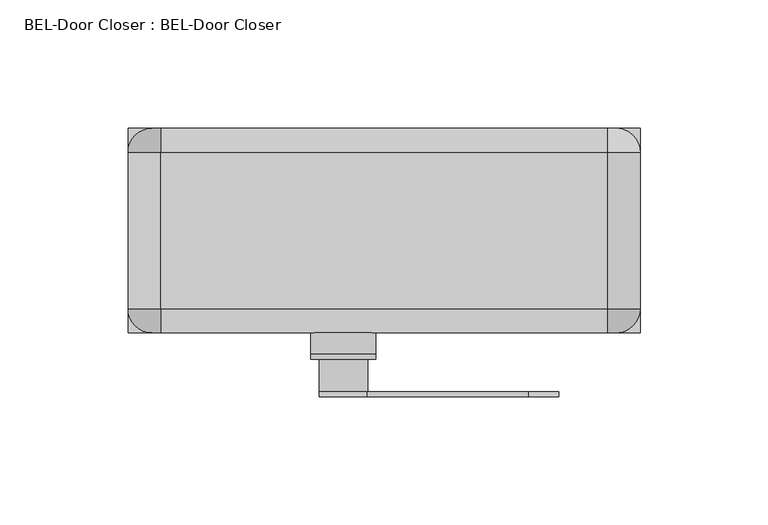
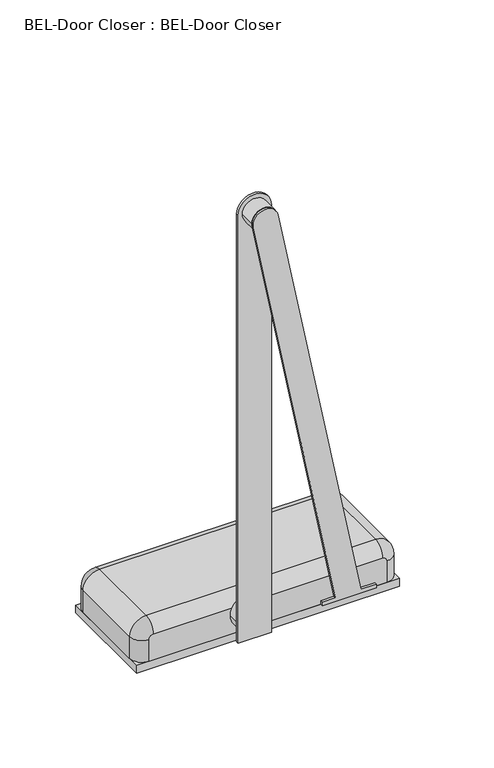
"""IFC4 building model written with IfcOpenShell, lengths in millimetres: proxy geometry, BEL-Door Closer : BEL-Door Closer."""

from ifc_helpers import new_model, si_unit, point, frame, frame_2d, origin, origin_with_axes, place, context, project, spatial, polyline, circle_curve, ellipse_curve, trimmed, segment, composite_curve, outline, extrude, source, transform, mapped, element, save
from ifc_brep_helpers import plane_surface, cylinder_surface, revolved_surface, advanced_brep


def bel_door_closer_bel_door_closer_f210e2f3(model_context):
    return source(origin(), model_context, "Body", "SolidModel", [
        extrude(outline(composite_curve([segment(trimmed(circle_curve(frame_2d((349.25, -273.05)), 9.525), [point((349.25, -282.575))], [point((349.25, -263.525))], False, "CARTESIAN"), True, "CONTINUOUS"), segment(trimmed(circle_curve(frame_2d((349.25, -273.05)), 9.525), [point((349.25, -263.525))], [point((349.25, -282.575))], False, "CARTESIAN"), True, "CONTINUOUS")], self_intersect=False)), frame((0.0, -45.1416667, 0.0), z_axis=(0.0, 1.0, 0.0), x_axis=(0.0, 0.0, 1.0)), (0.0, 0.0, 1.0), 12.5),
        extrude(outline(composite_curve([segment(trimmed(circle_curve(frame_2d((349.25, -273.0495842)), 9.5247276), [point((351.0696907, -263.7002975))], [point((347.4303363, -282.3988762))], False, "CARTESIAN"), True, "CONTINUOUS"), segment(polyline([(347.4303363, -282.3988762), (27.7698622, -220.1829834), (27.7542297, -229.9055371), (24.954228, -229.901035), (25.0199942, -188.9982584), (27.81999, -189.0027604), (27.8010501, -200.7822813), (351.0696907, -263.7002975)]), True, "CONTINUOUS")], self_intersect=False)), frame((0.0, -47.225, 0.0), z_axis=(0.0, 1.0, 0.0), x_axis=(0.0, 0.0, 1.0)), (0.0, 0.0, 1.0), 2.0833333),
        extrude(outline(composite_curve([segment(polyline([(5.475, -260.35), (349.25, -260.35)]), True, "CONTINUOUS"), segment(trimmed(circle_curve(frame_2d((349.25, -273.05)), 12.7), [point((349.25, -260.35))], [point((349.25, -285.75))], False, "CARTESIAN"), True, "CONTINUOUS"), segment(polyline([(349.25, -285.75), (5.475, -285.75), (5.475, -260.35)]), True, "CONTINUOUS")], self_intersect=False)), frame((0.0, -32.6416667, 0.0), z_axis=(0.0, 1.0, 0.0), x_axis=(0.0, 0.0, 1.0)), (0.0, 0.0, 1.0), 2.0833333),
        extrude(outline(composite_curve([segment(trimmed(circle_curve(frame_2d((21.35, -273.05)), 12.7), [point((21.35, -285.75))], [point((21.35, -260.35))], False, "CARTESIAN"), True, "CONTINUOUS"), segment(trimmed(circle_curve(frame_2d((21.35, -273.05)), 12.7), [point((21.35, -260.35))], [point((21.35, -285.75))], False, "CARTESIAN"), True, "CONTINUOUS")], self_intersect=False)), frame((0.0, -30.5583333, 0.0), z_axis=(0.0, 1.0, 0.0), x_axis=(0.0, 0.0, 1.0)), (0.0, 0.0, 1.0), 8.3333333),
        advanced_brep(
        [(-344.4875, -12.7, 36.35), (-169.8875, -12.7, 36.35), (-169.8875, 48.25, 36.35), (-344.4875, 48.25, 36.35), (-157.1875, -12.7, 6.35), (-166.7125, -22.225, 6.35), (-347.6625, -22.225, 6.35), (-357.1875, -12.7, 6.35), (-357.1875, 48.25, 6.35), (-347.6625, 57.775, 6.35), (-166.7125, 57.775, 6.35), (-157.1875, 48.25, 6.35), (-166.7125, -22.225, 23.65), (-169.8875, -22.225, 26.825), (-344.4875, -22.225, 26.825), (-347.6625, -22.225, 23.65), (-357.1875, -12.7, 23.65), (-357.1875, 48.25, 23.65), (-347.6625, 57.775, 23.65), (-344.4875, 57.775, 26.825), (-169.8875, 57.775, 26.825), (-166.7125, 57.775, 23.65), (-157.1875, 48.25, 23.65), (-157.1875, -12.7000056, 23.65)],
        [
            (0, 1),
            (1, 2),
            (2, 3),
            (3, 0),
            (4, 5, circle_curve(frame((-166.7125, -12.7, 6.35), z_axis=(0.0, 0.0, -1.0), x_axis=(-1.0, 0.0, 0.0)), 9.525)),
            (5, 6),
            (6, 7, circle_curve(frame((-347.6625, -12.7, 6.35), z_axis=(0.0, 0.0, -1.0), x_axis=(1.0, 0.0, 0.0)), 9.525)),
            (7, 8),
            (8, 9, circle_curve(frame((-347.6625, 48.25, 6.35), z_axis=(0.0, 0.0, -1.0), x_axis=(1.0, 0.0, 0.0)), 9.525)),
            (9, 10),
            (10, 11, circle_curve(frame((-166.7125, 48.25, 6.35), z_axis=(0.0, 0.0, -1.0), x_axis=(-1.0, 0.0, 0.0)), 9.525)),
            (11, 4),
            (5, 12),
            (12, 13, circle_curve(frame((-169.8875, -22.225, 23.65), z_axis=(0.0, -1.0, 0.0), x_axis=(0.0, 0.0, 1.0)), 3.175)),
            (13, 14),
            (14, 15, circle_curve(frame((-344.4875, -22.225, 23.65), z_axis=(0.0, -1.0, 0.0), x_axis=(-1.0, 0.0, 0.0)), 3.175)),
            (15, 6),
            (7, 16),
            (16, 17),
            (17, 8),
            (9, 18),
            (18, 19, circle_curve(frame((-344.4875, 57.775, 23.65), z_axis=(0.0, 1.0, 0.0), x_axis=(-1.0, 0.0, 0.0)), 3.175)),
            (19, 20),
            (20, 21, circle_curve(frame((-169.8875, 57.775, 23.65), z_axis=(0.0, 1.0, 0.0), x_axis=(0.0, 0.0, 1.0)), 3.175)),
            (21, 10),
            (11, 22),
            (22, 23),
            (23, 4),
            (3, 17, circle_curve(frame((-344.4875, 48.25, 23.65), z_axis=(0.0, -1.0, 0.0), x_axis=(1.0, 0.0, 0.0)), 12.7)),
            (16, 0, circle_curve(frame((-344.4875, -12.7, 23.65), z_axis=(0.0, 1.0, 0.0), x_axis=(1.0, 0.0, 0.0)), 12.7)),
            (1, 23, circle_curve(frame((-169.8875, -12.7, 23.65), z_axis=(0.0, 1.0, 0.0), x_axis=(1.0, 0.0, 0.0)), 12.7)),
            (22, 2, circle_curve(frame((-169.8875, 48.25, 23.65), z_axis=(0.0, -1.0, 0.0), x_axis=(1.0, 0.0, 0.0)), 12.7)),
            (15, 16, circle_curve(frame((-347.6625, -12.7, 23.65), z_axis=(0.0, 0.0, -1.0), x_axis=(1.0, 0.0, 0.0)), 9.525)),
            (17, 18, circle_curve(frame((-347.6625, 48.25, 23.65), z_axis=(0.0, 0.0, -1.0), x_axis=(1.0, 0.0, 0.0)), 9.525)),
            (14, 0, circle_curve(frame((-344.4875, -12.7, 26.825), z_axis=(-1.0, 0.0, 0.0), x_axis=(0.0, 0.0, -1.0)), 9.525)),
            (3, 19, circle_curve(frame((-344.4875, 48.25, 26.825), z_axis=(-1.0, 0.0, 0.0), x_axis=(0.0, 0.0, -1.0)), 9.525)),
            (13, 1, circle_curve(frame((-169.8875, -12.7, 26.825), z_axis=(-1.0, 0.0, 0.0), x_axis=(0.0, 0.0, -1.0)), 9.525)),
            (2, 20, circle_curve(frame((-169.8875, 48.25, 26.825), z_axis=(-1.0, 0.0, 0.0), x_axis=(0.0, 0.0, -1.0)), 9.525)),
            (12, 23, circle_curve(frame((-166.7125, -12.7, 23.65), z_axis=(0.0, 0.0, 1.0), x_axis=(-1.0, 0.0, 0.0)), 9.525)),
            (22, 21, circle_curve(frame((-166.7125, 48.25, 23.65), z_axis=(0.0, 0.0, 1.0), x_axis=(-1.0, 0.0, 0.0)), 9.525)),
        ],
        [
            plane_surface(frame((-357.1875, -22.225, 36.35), z_axis=(0.0, 0.0, 1.0), x_axis=(-1.0, 0.0, 0.0))),
            plane_surface(frame((-357.1875, -22.225, 6.35), z_axis=(0.0, 0.0, -1.0), x_axis=(1.0, 0.0, 0.0))),
            plane_surface(frame((-157.1875, -22.225, 36.35), z_axis=(0.0, -1.0, 0.0), x_axis=(0.0, 0.0, -1.0))),
            plane_surface(frame((-357.1875, -22.225, 36.35), z_axis=(-1.0, 0.0, 0.0), x_axis=(0.0, 0.0, -1.0))),
            plane_surface(frame((-357.1875, 57.775, 36.35), z_axis=(0.0, 1.0, 0.0), x_axis=(0.0, 0.0, -1.0))),
            plane_surface(frame((-157.1875, 57.775, 36.35), z_axis=(1.0, 0.0, 0.0), x_axis=(0.0, 0.0, -1.0))),
            cylinder_surface(frame((-344.4875, -22.225, 23.65), z_axis=(0.0, -1.0, 0.0), x_axis=(1.0, 0.0, 0.0)), 12.7),
            cylinder_surface(frame((-169.8875, 57.775, 23.65), z_axis=(0.0, -1.0, 0.0), x_axis=(1.0, 0.0, 0.0)), 12.7),
            cylinder_surface(frame((-347.6625, -12.7, 6.35), z_axis=(0.0, 0.0, 1.0), x_axis=(1.0, 0.0, 0.0)), 9.525),
            cylinder_surface(frame((-347.6625, 48.25, 6.35), z_axis=(0.0, 0.0, 1.0), x_axis=(1.0, 0.0, 0.0)), 9.525),
            revolved_surface(trimmed(ellipse_curve(frame((-347.6625, -12.7, 23.65), z_axis=(0.0, 0.0, 1.0), x_axis=(1.0, 0.0, 0.0)), 9.525, 9.525), [point((-357.1875, -12.7, 23.65))], [point((-347.6625, -22.225, 23.65))], True, "CARTESIAN"), (-344.4875, 57.775, 23.65), (0.0, -1.0, 0.0)),
            revolved_surface(trimmed(ellipse_curve(frame((-347.6625, 48.25, 23.65), z_axis=(0.0, 0.0, 1.0), x_axis=(1.0, 0.0, 0.0)), 9.525, 9.525), [point((-347.6625, 57.775, 23.65))], [point((-357.1875, 48.25, 23.65))], True, "CARTESIAN"), (-344.4875, 57.775, 23.65), (0.0, -1.0, 0.0)),
            cylinder_surface(frame((-344.4875, -12.7, 26.825), z_axis=(1.0, 0.0, 0.0), x_axis=(0.0, 0.0, -1.0)), 9.525),
            cylinder_surface(frame((-344.4875, 48.25, 26.825), z_axis=(1.0, 0.0, 0.0), x_axis=(0.0, 0.0, -1.0)), 9.525),
            revolved_surface(trimmed(ellipse_curve(frame((-169.8875, -12.7, 26.825), z_axis=(1.0, 0.0, 0.0), x_axis=(0.0, 0.0, -1.0)), 9.525, 9.525), [point((-169.8875, -12.7, 36.35))], [point((-169.8875, -22.225, 26.825))], True, "CARTESIAN"), (-169.8875, 57.775, 23.65), (0.0, -1.0, 0.0)),
            revolved_surface(trimmed(ellipse_curve(frame((-169.8875, 48.25, 26.825), z_axis=(1.0, 0.0, 0.0), x_axis=(0.0, 0.0, -1.0)), 9.525, 9.525), [point((-169.8875, 57.775, 26.825))], [point((-169.8875, 48.25, 36.35))], True, "CARTESIAN"), (-169.8875, 57.775, 23.65), (0.0, -1.0, 0.0)),
            cylinder_surface(frame((-166.7125, -12.7, 23.65), z_axis=(0.0, 0.0, -1.0), x_axis=(-1.0, 0.0, 0.0)), 9.525),
            cylinder_surface(frame((-166.7125, 48.25, 23.65), z_axis=(0.0, 0.0, -1.0), x_axis=(-1.0, 0.0, 0.0)), 9.525),
        ],
        [
            (0, [[1, 2, 3, 4]]),
            (1, [[5, 6, 7, 8, 9, 10, 11, 12]]),
            (2, [[13, 14, 15, 16, 17, -6]]),
            (3, [[18, 19, 20, -8]]),
            (4, [[21, 22, 23, 24, 25, -10]]),
            (5, [[26, 27, 28, -12]]),
            (6, [[29, -19, 30, -4]]),
            (7, [[31, -27, 32, -2]]),
            (8, [[-18, -7, -17, 33]]),
            (9, [[-21, -9, -20, 34]]),
            (10, [[-16, 35, -30, -33]]),
            (11, [[-29, 36, -22, -34]]),
            (12, [[-15, 37, -1, -35]]),
            (13, [[-3, 38, -23, -36]]),
            (14, [[-14, 39, -31, -37]]),
            (15, [[-32, 40, -24, -38]]),
            (16, [[-13, -5, -28, -39]]),
            (17, [[-26, -11, -25, -40]]),
        ],
    ),
        extrude(outline(polyline([(-157.1875, -22.225), (-357.1875, -22.225), (-357.1875, 57.775), (-157.1875, 57.775), (-157.1875, -22.225)])), origin_with_axes(), (0.0, 0.0, 1.0), 6.35),
    ])


if __name__ == "__main__":
    model = new_model("IFC4")
    model_context = context("Model", 3, world=origin())
    ifc_project = project(units=[si_unit("LENGTHUNIT", "METRE", prefix="MILLI")], contexts=[model_context])
    site = spatial("IfcSite", under=ifc_project)
    building = spatial("IfcBuilding", under=site)
    placement = place(None, origin())
    bel_door_closer_bel_door_closer_shape = bel_door_closer_bel_door_closer_f210e2f3(model_context)
    element("IfcBuildingElementProxy", 1, Name="BEL-Door Closer : BEL-Door Closer", ObjectType="BEL-Door Closer : BEL-Door Closer", at=placement, inside=building, context=model_context, shape_type="MappedRepresentation", body=[
        mapped(bel_door_closer_bel_door_closer_shape, transform((0.0, 0.0, 0.0), x_axis=(1.0, 0.0, 0.0), y_axis=(0.0, 1.0, 0.0), z_axis=(0.0, 0.0, 1.0))),
    ])
    save(model, "model.ifc")

# Revit data of these elements
# Type "BEL-Door Closer : BEL-Door Closer"
#   URL = "http://us.allegion.com/brands/falcon/Pages/default.aspx"
#   Standards Conformance = "as Specified"
#   Specification = ""
#   SpecWizard = ""
#   Send Message = "http://arcat.com/users.pl?action=UserEmail&company=Falcon+Lock&coid=32420&rep=114&fax=&mf="
#   Screw Pack Type = "as Specified"
#   Sales Information = "http://us.allegion.com/irst/Pages/contact_us.aspx"
#   Revision = "R1_02-2014"
#   Product Properties = ""
#   Product Data = "http://www.arcat.com/arcatcos/cos32/arc32420.html"
#   Model = "As Specified"
#   Manufacturer Website = "http://us.allegion.com/brands/falcon/Pages/default.aspx"
#   Manufacturer Phone = ""
#   Manufacturer Fax = ""
#   Manufacturer = "Falcon"
#   Keynote = "08710"
#   Installation-Fabrication = ""
#   Installation Phase = ""
#   Green Building-LEED = ""
#   Function Type = "as Specified"
#   Door Type = "as Specified"
#   Description = "Falcon Closer as Specified"
#   Copyright = "©Arcat Inc."
#   Construction Details = ""
#   Assembly Code = "C1020410"
#   originlocate [instance default] = 0' - 0"
#   locatearm [instance default] = 0' - 0 1/2"
#   Unit Width = 0' - 7.87402"
#   Unit Height = 0' - 3.14961"
#   Unit Depth = 0' - 1.1811"
#   Plate Thickness = 0' - 0 1/4"
#   Offset from Edge of Frame_Closer Arm [instance default] = 0' - 7"
#   Offset from Edge of Door_Closer Case [instance default] = 0' - 3 15/16"
#   Offset for Plate [instance default] = 0' - 0"
#   Reveal Between Door and Frame_Right [instance default] = 0' - 0 1/4"
#   Reveal Between Door and Frame_Left [instance default] = 0' - 0 1/4"
#   Door Leaf Width [instance default] = 3' - 0"
#   Door Leaf Top Reveal [instance default] = 0' - 0 1/4"
#   Door Leaf Thickness [instance default] = 0' - 0"
#   Closer Case Side Offset = 0' - 3 15/16"
#   Closer Arm Offset = 0' - 7"
#   Arm Width = 1' - 2"
#   Arm Height = 0' - 1 5/8"
#   Arm Extension [instance default] = 0' - 0"
#   Arm Depth = 1' - 2"
#   ActualArm Height [instance default] = 0' - 1 7/8"
#   ActualArm Depth [instance default] = 1' - 2"
#   Warranty Duration (Years) = 0
#   RH Hinge [instance default] = no
#   Maintenance Schedule (Months) = 0
#   LH Hinge [instance default] = yes
#   Include Mounting Plate [instance default] = no
#   Expected Lifespan (Years) = 0
#   Closer on Door Surface = yes
#   Closer on Door Frame = no
#   Arm Below Closer = no
#   Arm Above Closer = yes
#   Cover Material [instance default] = Metal - IR - Satin Chrome
#   Arm Type = element 418778
#   Arm Material [instance default] = Metal - IR - Satin Chrome
#   Default Elevation = 0
# Element 1 (IfcBuildingElementProxy, "BEL-Door Closer : BEL-Door Closer")
#   Offset for Plate = 0' - 0 1/4"
#   ActualArm Depth = 1' - 2 1/4"
#   Include Mounting Plate = yes
#   Materials on its faces: "Metal - IR - Satin Chrome"
# Materials
#   "Metal - IR - Satin Chrome": colour RGB 244 244 244, transparency 0, Cost = 0
